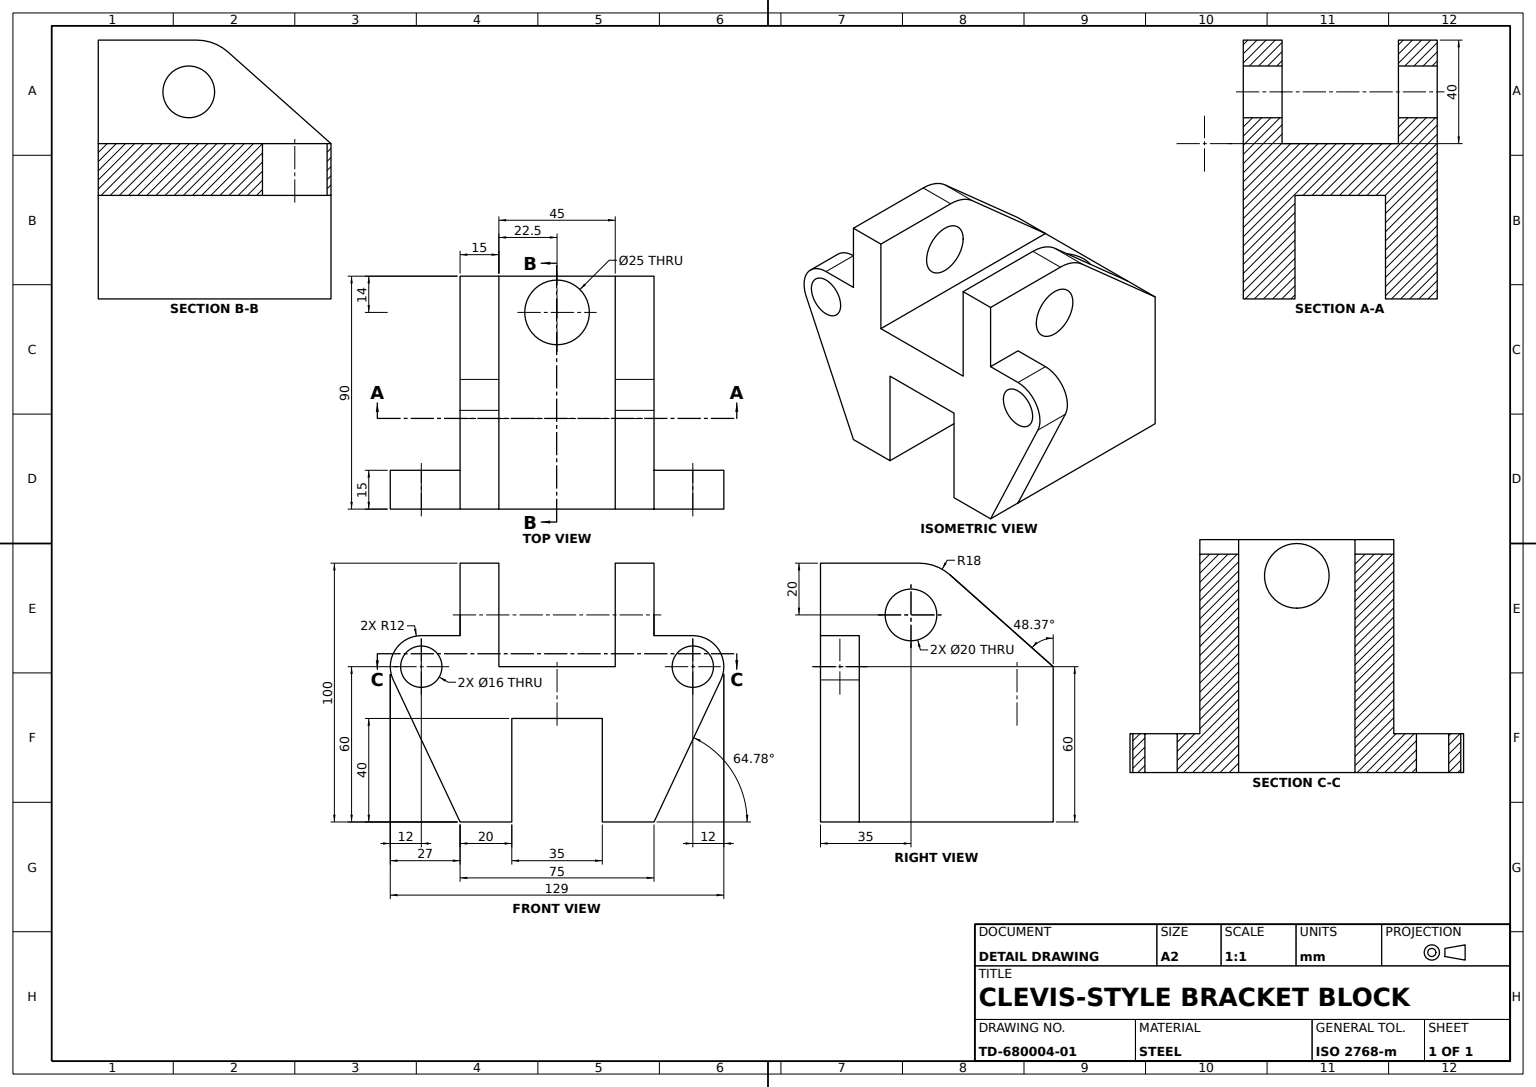
SolidWorks part; units mm, degrees
material "Plain Carbon Steel"
ref_plane "Front Plane" through (0, 0, 0) normal (0, 0, 1) x (1, 0, 0)
ref_plane "Top Plane" through (0, 0, 0) normal (0, 1, 0) x (1, 0, 0)
ref_plane "Right Plane" through (0, 0, 0) normal (1, 0, 0) x (0, 0, -1)
sketch "Base Profile Sketch" plane through (0, 0, 0) normal (1, 0, 0) x (0, 0, -1)
  line L0 (0, 0) -> (90, 0)
  line L1 (90, 0) -> (90, 60)
  line L2 (0, 0) -> (0, 100)
  line L3 (0, 100) -> (45, 100)
  line L4 (45, 100) -> (90, 60)
  dimension "D1" = 90
  dimension "D2" = 60
  dimension "D3" = 100
  dimension "D4" = 45
extrude "Base Block" add sketch "Base Profile Sketch" against normal blind 75
sketch "Bottom Notch Sketch" plane through (0, 0, -90) normal (0, 0, -1) x (-1, 0, 0)
  line L0 (75, 0) -> (0, 0) construction
  line L1 (20, 0) -> (55, 0)
  line L2 (20, 0) -> (20, 40)
  line L3 (20, 40) -> (55, 40)
  line L4 (55, 0) -> (55, 40)
  line L5 (75, 60) -> (0, 60) construction
  dimension "D1" = 20
  dimension "D2" = 20
  dimension "D3" = 20
extrude "Bottom Notch" cut sketch "Bottom Notch Sketch" against normal through all
sketch "Top Slot Sketch" plane through (0, 100, 0) normal (0, 1, 0) x (1, 0, 0)
  line L0 (-75, 0) -> (0, 0) construction
  line L1 (-60, 0) -> (-15, 0)
  line L2 (-60, 0) -> (-60, 90)
  line L3 (-60, 90) -> (-15, 90)
  line L4 (-15, 0) -> (-15, 90)
  line L5 (-75, 90) -> (0, 90) construction
  dimension "D1" = 15
  dimension "D2" = 15
extrude "Top Slot" cut sketch "Top Slot Sketch" against normal blind 40
fillet "Edge Fillet R18" radius 18 2 edges at (-7.5, 100, -45) (-67.5, 100, -45)
sketch "Cross Hole Sketch" plane through (0, 0, 0) normal (1, 0, 0) x (0, 0, -1)
  line L0 (38.1564, 100) -> (0, 100) construction
  line L1 (0, 100) -> (0, 0) construction
  circle A0 centre (35, 80) radius 10
  dimension "D1" = 20
  dimension "D2" = 20
  dimension "D3" = 35
extrude "Cross Hole" cut sketch "Cross Hole Sketch" against normal through all
sketch "Pin Hole Sketch" plane through (0, 60, 0) normal (0, 1, 0) x (1, 0, 0)
  line L0 (-15, 90) -> (-60, 90) construction
  circle A0 centre (-37.5, 76) radius 12.5
  dimension "D1" = 25
  dimension "D2" = 22.5
  dimension "D3" = 14
extrude "Pin Hole" cut sketch "Pin Hole Sketch" against normal blind 40
sketch "Side Lugs Sketch" plane through (0, 0, 0) normal (0, 0, 1) x (1, 0, 0)
  line L0 (0, 100) -> (0, 0) construction
  line L1 (-20, 0) -> (0, 0) construction
  line L2 (15, 72) -> (0, 72)
  line L3 (0, 72) -> (0, 0)
  line L4 (0, 0) -> (25.8558, 54.8861)
  line L5 (-75, 100) -> (-75, 0) construction
  line L6 (-90, 72) -> (-75, 72)
  line L7 (-75, 72) -> (-75, 0)
  line L8 (-75, 0) -> (-100.8558, 54.8861)
  arc A0 (25.8558, 54.8861) -> (15, 72) centre (15, 60) ccw
  circle A1 centre (15, 60) radius 8
  arc A2 (-90, 72) -> (-100.8558, 54.8861) centre (-90, 60) ccw
  circle A3 centre (-90, 60) radius 8
  dimension "D1" = 24
  dimension "D4" = 16
  dimension "D5" = 24
  dimension "D9" = 16
  dimension "D2" = 15
  dimension "D3" = 60
  dimension "D6" = 60
  dimension "D7" = 15
  dimension "D8" = 15
extrude "Side Lugs" add sketch "Side Lugs Sketch" against normal blind 15
